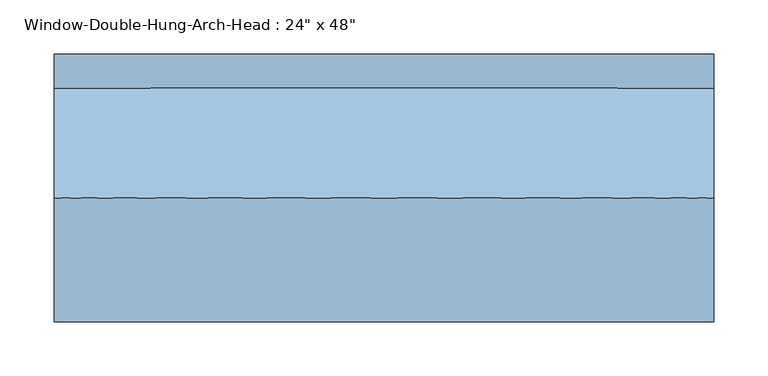
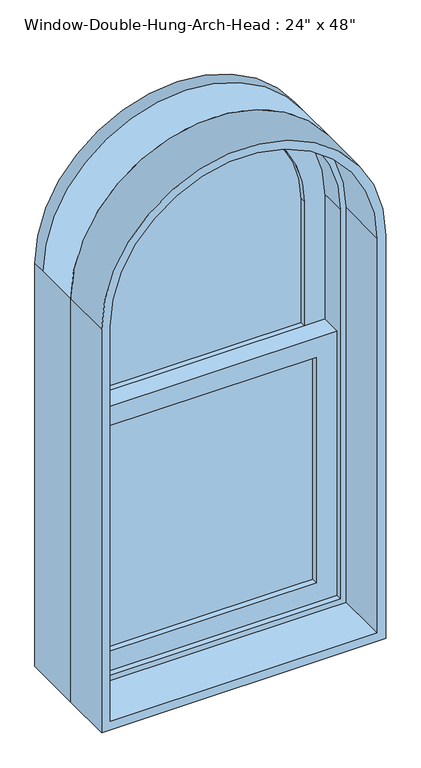
"""IFC4 building model written with IfcOpenShell, lengths in millimetres: window geometry."""

from ifc_helpers import new_model, si_unit, point, frame, frame_2d, origin, place, context, project, spatial, polyline, circle_curve, trimmed, segment, composite_curve, outline, extrude, source, transform, mapped, element, save
from ifc_brep_helpers import plane_surface, cylinder_surface, revolved_surface, advanced_brep


def window_777a1d98(model_context):
    return source(origin(), model_context, "Body", "SolidModel", [
        extrude(outline(composite_curve([segment(polyline([(1828.8, -304.8), (914.4, -304.8), (914.4, 304.8), (1828.8, 304.8)]), True, "CONTINUOUS"), segment(trimmed(circle_curve(frame_2d((1828.8, 0.0)), 304.8), [point((1828.8, 304.8))], [point((1828.8, -304.8))], False, "CARTESIAN"), True, "CONTINUOUS")], self_intersect=False), holes=[composite_curve([segment(trimmed(circle_curve(frame_2d((1828.8, 0.0)), 285.75), [point((1828.8, -285.75))], [point((1828.8, 285.75))], True, "CARTESIAN"), True, "CONTINUOUS"), segment(polyline([(1828.8, 285.75), (933.45, 285.75), (933.45, -285.75), (1828.8, -285.75)]), True, "CONTINUOUS")], self_intersect=False)]), frame((0.0, -114.3, 0.0), z_axis=(0.0, 1.0, 0.0), x_axis=(0.0, 0.0, 1.0)), (0.0, 0.0, 1.0), 114.3),
        extrude(outline(polyline([(1546.225, -273.05), (946.15, -273.05), (946.15, 273.05), (1546.225, 273.05), (1546.225, -273.05)]), holes=[polyline([(1501.775, 228.6), (990.6, 228.6), (990.6, -228.6), (1501.775, -228.6), (1501.775, 228.6)])]), frame((0.0, 12.7, 0.0), z_axis=(0.0, 1.0, 0.0), x_axis=(0.0, 0.0, 1.0)), (0.0, 0.0, 1.0), 44.45),
        extrude(outline(polyline([(228.6, 44.45), (228.6, 38.1), (-228.6, 38.1), (-228.6, 44.45), (228.6, 44.45)])), frame((0.0, 0.0, 990.6), z_axis=(0.0, 0.0, 1.0), x_axis=(1.0, 0.0, 0.0)), (0.0, 0.0, 1.0), 511.175),
        extrude(outline(polyline([(-228.6, 31.75), (228.6, 31.75), (228.6, 25.4), (-228.6, 25.4), (-228.6, 31.75)])), frame((0.0, 0.0, 990.6), z_axis=(0.0, 0.0, 1.0), x_axis=(1.0, 0.0, 0.0)), (0.0, 0.0, 1.0), 511.175),
        extrude(outline(composite_curve([segment(polyline([(1828.8, -228.6), (1546.225, -228.6), (1546.225, 228.6), (1828.8, 228.6)]), True, "CONTINUOUS"), segment(trimmed(circle_curve(frame_2d((1828.8, 0.0)), 228.6), [point((1828.8, 228.6))], [point((1828.8, -228.6))], False, "CARTESIAN"), True, "CONTINUOUS")], self_intersect=False)), frame((0.0, 82.55, 0.0), z_axis=(0.0, 1.0, 0.0), x_axis=(0.0, 0.0, 1.0)), (0.0, 0.0, 1.0), 6.35),
        extrude(outline(composite_curve([segment(polyline([(1828.8, -228.6), (1546.225, -228.6), (1546.225, 228.6), (1828.8, 228.6)]), True, "CONTINUOUS"), segment(trimmed(circle_curve(frame_2d((1828.8, 0.0)), 228.6), [point((1828.8, 228.6))], [point((1828.8, -228.6))], False, "CARTESIAN"), True, "CONTINUOUS")], self_intersect=False)), frame((0.0, 69.85, 0.0), z_axis=(0.0, 1.0, 0.0), x_axis=(0.0, 0.0, 1.0)), (0.0, 0.0, 1.0), 6.35),
        advanced_brep(
        [(-304.8, 133.35, 1828.8), (-304.8, 133.35, 914.4), (-304.8, 0.0, 914.4), (-304.8, 0.0, 1828.8), (-304.8, 101.6, 1828.8), (-273.05, 0.0, 1828.8), (-273.05, 0.0, 946.15), (-273.05, 133.35, 946.15), (-273.05, 133.35, 1828.8), (-273.05, 101.6, 1828.8), (304.8, 133.35, 914.4), (304.8, 0.0, 914.4), (273.05, 0.0, 946.15), (273.05, 133.35, 946.15), (304.8, 133.35, 1828.8), (304.8, 101.6, 1828.8), (304.8, 0.0, 1828.8), (273.05, 0.0, 1828.8), (273.05, 101.6, 1828.8), (273.05, 133.35, 1828.8), (0.0, 101.6, 2133.6)],
        [
            (0, 1),
            (1, 2),
            (2, 3),
            (3, 4),
            (4, 0),
            (5, 6),
            (6, 7),
            (7, 8),
            (8, 9),
            (9, 5),
            (1, 10),
            (10, 11),
            (11, 2),
            (6, 12),
            (12, 13),
            (13, 7),
            (10, 14),
            (14, 15),
            (15, 16),
            (16, 11),
            (12, 17),
            (17, 18),
            (18, 19),
            (19, 13),
            (3, 16, circle_curve(frame((0.0, 0.0, 1828.8), z_axis=(0.0, 1.0, 0.0), x_axis=(1.0, 0.0, 0.0)), 304.8)),
            (15, 20, circle_curve(frame((0.0, 101.6, 1828.8), z_axis=(0.0, -1.0, 0.0), x_axis=(1.0, 0.0, 0.0)), 304.8)),
            (20, 4, circle_curve(frame((0.0, 101.6, 1828.8), z_axis=(0.0, -1.0, 0.0), x_axis=(1.0, 0.0, 0.0)), 304.8)),
            (5, 17, circle_curve(frame((0.0, 0.0, 1828.8), z_axis=(0.0, 1.0, 0.0), x_axis=(1.0, 0.0, 0.0)), 273.05)),
            (9, 18, circle_curve(frame((0.0, 101.6, 1828.8), z_axis=(0.0, 1.0, 0.0), x_axis=(1.0, 0.0, 0.0)), 273.05)),
            (0, 14, circle_curve(frame((0.0, 133.35, 1828.8), z_axis=(0.0, 1.0, 0.0), x_axis=(-1.0, 0.0, 0.0)), 304.8)),
            (19, 8, circle_curve(frame((0.0, 133.35, 1828.8), z_axis=(0.0, -1.0, 0.0), x_axis=(-1.0, 0.0, 0.0)), 273.05)),
        ],
        [
            plane_surface(frame((-304.8, 133.35, 1828.8), z_axis=(-1.0, 0.0, 0.0), x_axis=(0.0, 0.0, -1.0))),
            plane_surface(frame((-273.05, 0.0, 1828.8), z_axis=(1.0, 0.0, 0.0), x_axis=(0.0, 0.0, -1.0))),
            plane_surface(frame((-304.8, 133.35, 914.4), z_axis=(0.0, 0.0, -1.0), x_axis=(1.0, 0.0, 0.0))),
            plane_surface(frame((-273.05, 0.0, 946.15), z_axis=(0.0, 0.0, 1.0), x_axis=(1.0, 0.0, 0.0))),
            plane_surface(frame((304.8, 133.35, 914.4), z_axis=(1.0, 0.0, 0.0), x_axis=(0.0, 0.0, 1.0))),
            plane_surface(frame((273.05, 0.0, 946.15), z_axis=(-1.0, 0.0, 0.0), x_axis=(0.0, 0.0, 1.0))),
            cylinder_surface(frame((0.0, 101.6, 1828.8), z_axis=(0.0, -1.0, 0.0), x_axis=(1.0, 0.0, 0.0)), 304.8),
            plane_surface(frame((0.0, 0.0, 1828.8), z_axis=(0.0, -1.0, 0.0), x_axis=(1.0, 0.0, 0.0))),
            revolved_surface(polyline([(273.05, 0.0, 1828.8), (273.05, 101.6, 1828.8)]), (0.0, 101.6, 1828.8), (0.0, -1.0, 0.0)),
            plane_surface(frame((0.0, 133.35, 1828.8), z_axis=(0.0, 1.0, 0.0), x_axis=(1.0, 0.0, 0.0))),
            cylinder_surface(frame((0.0, 133.35, 1828.8), z_axis=(0.0, 1.0, 0.0), x_axis=(-1.0, 0.0, 0.0)), 304.8),
            revolved_surface(polyline([(-273.05, 133.35, 1828.8), (-273.05, 101.6, 1828.8)]), (0.0, 133.35, 1828.8), (0.0, 1.0, 0.0)),
        ],
        [
            (0, [[1, 2, 3, 4, 5]]),
            (1, [[6, 7, 8, 9, 10]]),
            (2, [[-2, 11, 12, 13]]),
            (3, [[-7, 14, 15, 16]]),
            (4, [[-12, 17, 18, 19, 20]]),
            (5, [[-15, 21, 22, 23, 24]]),
            (6, [[25, -19, 26, 27, -4]]),
            (7, [[-3, -13, -20, -25], [-6, 28, -21, -14]]),
            (8, [[-28, -10, 29, -22]]),
            (9, [[-1, 30, -17, -11], [-24, 31, -8, -16]]),
            (10, [[-30, -5, -27, -26, -18]]),
            (11, [[-31, -23, -29, -9]]),
        ],
    ),
        advanced_brep(
        [(-273.05, 101.6, 1828.8), (-273.05, 101.6, 1501.775), (-273.05, 57.15, 1501.775), (-273.05, 57.15, 1828.8), (-273.05, 88.9, 1828.8), (-228.6, 57.15, 1828.8), (-228.6, 57.15, 1546.225), (-228.6, 101.6, 1546.225), (-228.6, 101.6, 1828.8), (-228.6, 88.9, 1828.8), (273.05, 101.6, 1501.775), (273.05, 57.15, 1501.775), (228.6, 57.15, 1546.225), (228.6, 101.6, 1546.225), (273.05, 101.6, 1828.8), (273.05, 88.9, 1828.8), (273.05, 57.15, 1828.8), (228.6, 57.15, 1828.8), (228.6, 88.9, 1828.8), (228.6, 101.6, 1828.8), (0.0, 88.9, 2101.85)],
        [
            (0, 1),
            (1, 2),
            (2, 3),
            (3, 4),
            (4, 0),
            (5, 6),
            (6, 7),
            (7, 8),
            (8, 9),
            (9, 5),
            (1, 10),
            (10, 11),
            (11, 2),
            (6, 12),
            (12, 13),
            (13, 7),
            (10, 14),
            (14, 15),
            (15, 16),
            (16, 11),
            (12, 17),
            (17, 18),
            (18, 19),
            (19, 13),
            (0, 14, circle_curve(frame((0.0, 101.6, 1828.8), z_axis=(0.0, 1.0, 0.0), x_axis=(-1.0, 0.0, 0.0)), 273.05)),
            (19, 8, circle_curve(frame((0.0, 101.6, 1828.8), z_axis=(0.0, -1.0, 0.0), x_axis=(-1.0, 0.0, 0.0)), 228.6)),
            (3, 16, circle_curve(frame((0.0, 57.15, 1828.8), z_axis=(0.0, 1.0, 0.0), x_axis=(1.0, 0.0, 0.0)), 273.05)),
            (15, 20, circle_curve(frame((0.0, 88.9, 1828.8), z_axis=(0.0, -1.0, 0.0), x_axis=(1.0, 0.0, 0.0)), 273.05)),
            (20, 4, circle_curve(frame((0.0, 88.9, 1828.8), z_axis=(0.0, -1.0, 0.0), x_axis=(1.0, 0.0, 0.0)), 273.05)),
            (5, 17, circle_curve(frame((0.0, 57.15, 1828.8), z_axis=(0.0, 1.0, 0.0), x_axis=(1.0, 0.0, 0.0)), 228.6)),
            (9, 18, circle_curve(frame((0.0, 88.9, 1828.8), z_axis=(0.0, 1.0, 0.0), x_axis=(1.0, 0.0, 0.0)), 228.6)),
        ],
        [
            plane_surface(frame((-273.05, 101.6, 1828.8), z_axis=(-1.0, 0.0, 0.0), x_axis=(0.0, 0.0, -1.0))),
            plane_surface(frame((-228.6, 57.15, 1828.8), z_axis=(1.0, 0.0, 0.0), x_axis=(0.0, 0.0, -1.0))),
            plane_surface(frame((-273.05, 101.6, 1501.775), z_axis=(0.0, 0.0, -1.0), x_axis=(1.0, 0.0, 0.0))),
            plane_surface(frame((-228.6, 57.15, 1546.225), z_axis=(0.0, 0.0, 1.0), x_axis=(1.0, 0.0, 0.0))),
            plane_surface(frame((273.05, 101.6, 1501.775), z_axis=(1.0, 0.0, 0.0), x_axis=(0.0, 0.0, 1.0))),
            plane_surface(frame((228.6, 57.15, 1546.225), z_axis=(-1.0, 0.0, 0.0), x_axis=(0.0, 0.0, 1.0))),
            plane_surface(frame((0.0, 101.6, 1828.8), z_axis=(0.0, 1.0, 0.0), x_axis=(1.0, 0.0, 0.0))),
            cylinder_surface(frame((0.0, 101.6, 1828.8), z_axis=(0.0, -1.0, 0.0), x_axis=(1.0, 0.0, 0.0)), 273.05),
            plane_surface(frame((0.0, 57.15, 1828.8), z_axis=(0.0, -1.0, 0.0), x_axis=(1.0, 0.0, 0.0))),
            revolved_surface(polyline([(228.6, 57.15, 1828.8), (228.6, 88.9, 1828.8)]), (0.0, 101.6, 1828.8), (0.0, -1.0, 0.0)),
            cylinder_surface(frame((0.0, 101.6, 1828.8), z_axis=(0.0, 1.0, 0.0), x_axis=(-1.0, 0.0, 0.0)), 273.05),
            revolved_surface(polyline([(-228.6, 101.6, 1828.8), (-228.6, 88.9, 1828.8)]), (0.0, 101.6, 1828.8), (0.0, 1.0, 0.0)),
        ],
        [
            (0, [[1, 2, 3, 4, 5]]),
            (1, [[6, 7, 8, 9, 10]]),
            (2, [[-2, 11, 12, 13]]),
            (3, [[-7, 14, 15, 16]]),
            (4, [[-12, 17, 18, 19, 20]]),
            (5, [[-15, 21, 22, 23, 24]]),
            (6, [[-1, 25, -17, -11], [-24, 26, -8, -16]]),
            (7, [[27, -19, 28, 29, -4]]),
            (8, [[-3, -13, -20, -27], [-6, 30, -21, -14]]),
            (9, [[-30, -10, 31, -22]]),
            (10, [[-25, -5, -29, -28, -18]]),
            (11, [[-26, -23, -31, -9]]),
        ],
    ),
    ])


if __name__ == "__main__":
    model = new_model("IFC4")
    model_context = context("Model", 3, world=origin())
    ifc_project = project(units=[si_unit("LENGTHUNIT", "METRE", prefix="MILLI")], contexts=[model_context])
    site = spatial("IfcSite", under=ifc_project)
    building = spatial("IfcBuilding", under=site)
    placement = place(None, origin())
    window_shape = window_777a1d98(model_context)
    element("IfcWindow", 1, ObjectType="Window-Double-Hung-Arch-Head : 24\" x 48\"", at=placement, inside=building, context=model_context, shape_type="MappedRepresentation", body=[
        mapped(window_shape, transform((0.0, 0.0, 0.0), x_axis=(1.0, 0.0, 0.0), y_axis=(0.0, 1.0, 0.0), z_axis=(0.0, 0.0, 1.0))),
    ])
    save(model, "model.ifc")

# Revit data of these elements
# Type "Window-Double-Hung-Arch-Head : 24\" x 48\""
#   Type Mark = "19"
#   Fire Rating = "0.5h"
#   Construction Type Id = "DG-DR"
#   Assembly Code = "B2020100"
#   Analytic Construction = "Double glazing - domestic"
#   Wall Thickness [instance default] = 0' - 6"
#   Window Inset [instance default] = 0' - 0"
#   Visual Light Transmittance = 0.81
#   Thermal Resistance (R) = 1.8146 (h·ft²·°F)/BTU
#   Solar Heat Gain Coefficient = 0.76
#   Muntin Width = 1' - 6"
#   Muntin Height = 1' - 8 1/8"
#   Interior Wall Closure [instance default] = 0' - 1 1/2"
#   Rough Width = 2' - 0 1/2"
#   Rough Height = 4' - 0 1/2"
#   Half Width = 1' - 0"
#   Frame Extension [instance default] = 0' - 1 1/4"
#   Exterior Wall Closure [instance default] = 0' - 0 1/2"
#   Extension Jamb [instance default] = 0' - 1 1/2"
#   Heat Transfer Coefficient (U) = 0.5511 BTU/(h·ft²·°F)
#   Height = 4' - 0"
#   Width = 2' - 0"
#   Top Muntin Visibility = yes
#   Indicator Visibility [instance default] = yes
#   Extension Jamb Visibility [instance default] = yes
#   Interior Trim Visibility [instance default] = yes
#   Exterior Trim Visibility [instance default] = yes
#   Define Thermal Properties by = 1
#   Bottom Muntin Visibility = yes
#   Muntin Pattern = Muntin Pattern_2x2 : Muntin Pattern_2x2
#   Interior Trim Material = Wood - Stained
#   Interior Trim = Trim-Window-Interior-Arch-Hung : Picture Frame
#   Exterior Trim Material = Clad - White
#   Exterior Trim = Trim-Window-Exterior-Arch-Hung : with Sill
#   Glass Panel Material = Glass
#   Exterior Frame Material = Clad - White
#   Interior Frame Material = Wood - Stained
#   Wall Closure = (empty or 0)
# Element 1 (IfcWindow, "Window-Double-Hung-Arch-Head : 24\" x 48\"")
#   Wall Thickness = 0' - 9"
#   Extension Jamb = 0' - 4 1/2"
#   Materials on its faces: "Wood - Stained", "Glass", "Clad - White"
# Materials
#   "Wood - Stained": class "Wood", colour RGB 224 178 126, transparency 0, Cost = 0
#   "Clad - White": class "Wood", colour RGB 242 242 238, transparency 0, Cost = 0
#   "Glass": class "Glass", colour RGB 0 128 192, transparency 0.75, Description = "Soda Lime Glass", Cost = 0
